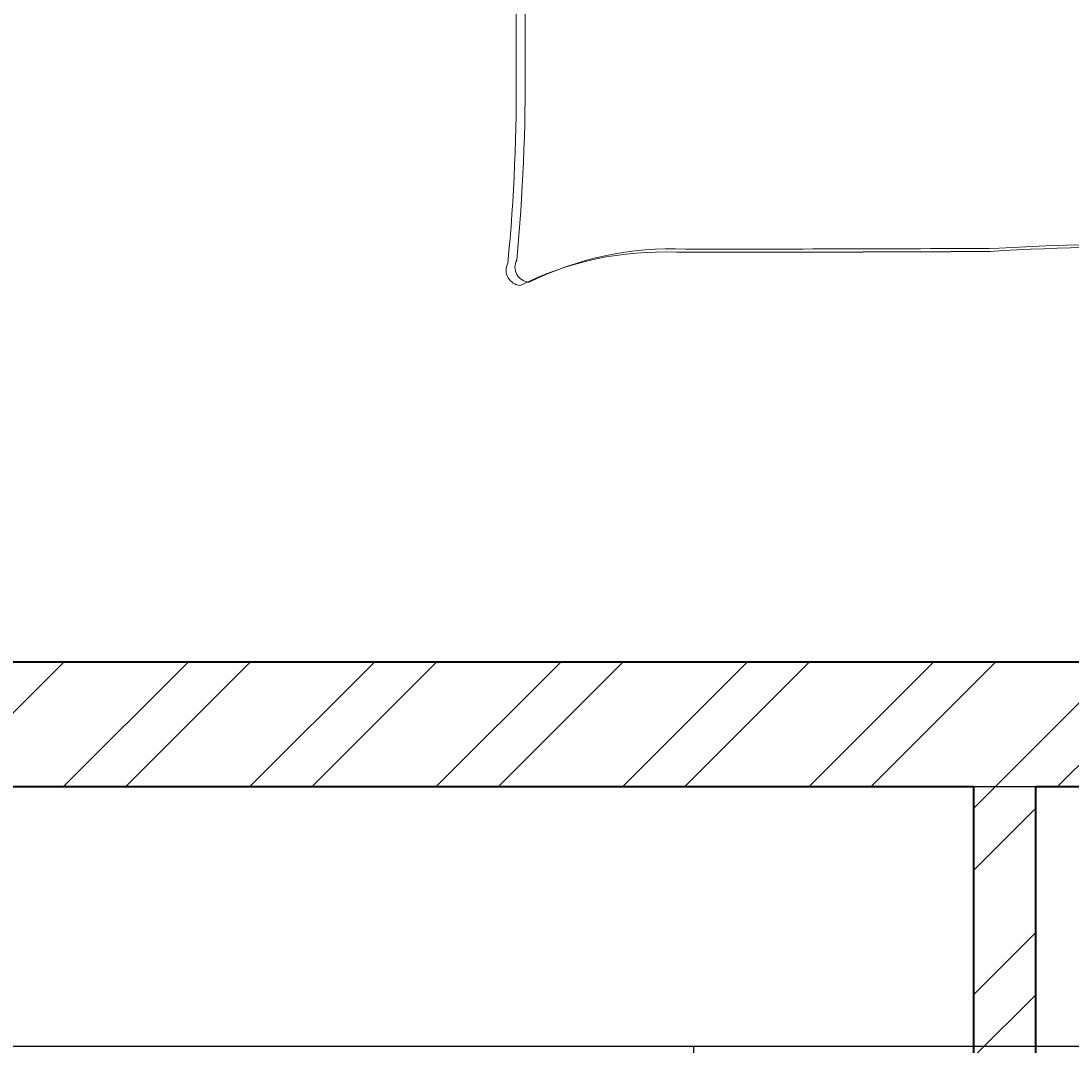
# Model space of a CAD drawing. Units: inches. Extents: x 1601 to 2297, y 1496 to 2631.
# Tile 29 of 57: x 2109 to 2185, y 2067 to 2141. Entities that reach past the tile are written whole.
import ezdxf

# ---------------------------------------------------------------- set-up
doc = ezdxf.new("R2010")
doc.units = ezdxf.units.IN
for name, color, linetype, lineweight in [('A-ANNO-DIMS', 2, 'Continuous', 18), ('A-FURN', 8, 'Continuous', 18), ('A-WALL', 7, 'Continuous', 40), ('A-WALL-PATT', 215, 'Continuous', 13)]:
    doc.layers.add(name, color=color, linetype=linetype, lineweight=lineweight)
doc.styles.get("Standard").update_dxf_attribs({"font": 'arial.ttf'})
doc.dimstyles.get("Standard").update_dxf_attribs({"dimtxt": 0.18, "dimasz": 0.18, "dimexe": 0.18, "dimexo": 0.0625, "dimgap": 0.09, "dimtad": 0, "dimtih": 1, "dimtoh": 1, "dimdec": 4, "dimzin": 0, "dimdsep": 46, "dimtxsty": 'Standard', "dimcen": 0.09, "dimadec": 0, "dimazin": 0, "dimtfac": 1, "dimtdec": 4, "dimtofl": 0, "dimtmove": 0, "dimatfit": 3, "dimfxl": 1, "dimtolj": 1, "dimtzin": 0, "dimarcsym": 0})

# ---------------------------------------------------------------- blocks, each defined once
blk = doc.blocks.new('BED-DOUBLE')
for p, q in [((30.13, 53.175), (28.385, 53.096, 3.871)), ((30.13, 53.175), (28.385, 53.096, 3.871)), ((30.13, 53.175), (28.385, 53.096, 3.871)), ((30.13, 53.175), (28.385, 53.096, 3.871)), ((27.746, 52.867), (24.495, 49.162)), ((27.746, 52.867), (24.495, 49.162)), ((27.746, 52.867), (24.495, 49.162)), ((27.746, 52.867), (24.495, 49.162)), ((28.385, 53.096), (25.135, 49.39)), ((28.385, 53.096), (25.135, 49.39)), ((28.385, 53.096), (25.135, 49.39)), ((28.385, 53.096), (25.135, 49.39)), ((29.49, 52.947), (27.746, 52.867, 3.871)), ((29.49, 52.947), (27.746, 52.867, 3.871)), ((29.49, 52.947), (27.746, 52.867, 3.871)), ((29.49, 52.947), (27.746, 52.867, 3.871)), ((28.365, 51.33), (27.746, 52.867)), ((28.365, 51.33), (27.746, 52.867)), ((28.365, 51.33), (27.746, 52.867)), ((28.365, 51.33), (27.746, 52.867)), ((29.004, 51.559), (28.385, 53.096)), ((29.004, 51.558), (28.385, 53.096)), ((29.004, 51.559), (28.385, 53.096)), ((29.004, 51.558), (28.385, 53.096)), ((0, 51.494), (0.639, 51.493)), ((0, 3.475), (0, 51.494)), ((0, 51.494), (0.639, 51.493)), ((0, 3.475), (0, 51.494)), ((0, 51.265), (26.61, 51.265)), ((0, 51.265), (26.61, 51.265)), ((0, 51.265), (26.61, 51.265)), ((0, 51.265), (26.61, 51.265)), ((0.639, 51.494), (27.249, 51.494)), ((0.639, 51.494), (27.249, 51.494)), ((0.639, 51.493), (27.249, 51.493)), ((0.639, 51.493), (27.249, 51.493)), ((1.533, 3.475), (1.533, 51.265)), ((1.533, 3.475), (1.533, 51.265)), ((1.533, 3.475), (1.533, 51.265)), ((1.533, 3.475), (1.533, 51.265)), ((2.173, 3.703), (2.173, 51.494)), ((2.173, 3.703), (2.173, 51.494)), ((2.173, 3.703), (2.173, 51.493)), ((2.173, 3.703), (2.173, 51.493)), ((17.212, 50.926), (14.073, 50.151)), ((17.212, 50.926), (14.073, 50.151)), ((17.212, 50.926), (14.073, 50.151)), ((17.212, 50.926), (14.073, 50.151)), ((16.808, 45.795), (17.212, 50.926)), ((16.808, 45.794), (17.212, 50.926)), ((16.808, 45.795), (17.212, 50.926)), ((16.808, 45.794), (17.212, 50.926)), ((28.055, 48.233), (28.365, 51.33)), ((28.055, 48.233), (28.365, 51.33)), ((28.055, 48.233), (28.365, 51.33)), ((28.055, 48.233), (28.365, 51.33)), ((28.695, 48.461), (29.004, 51.559)), ((28.695, 48.461), (29.004, 51.559)), ((28.695, 48.461), (29.004, 51.558)), ((28.695, 48.461), (29.004, 51.558)), ((2.557, 50.112), (2.46, 44.709)), ((2.557, 50.112), (2.46, 44.709)), ((2.557, 50.111), (2.46, 44.709)), ((2.557, 50.111), (2.46, 44.709)), ((2.557, 50.112), (5.768, 49.733)), ((2.557, 50.112), (5.768, 49.733)), ((2.557, 50.111), (5.768, 49.733)), ((2.557, 50.111), (5.768, 49.733)), ((3.196, 50.34), (3.099, 44.938)), ((3.196, 50.34), (3.099, 44.938)), ((3.196, 50.34), (3.099, 44.938)), ((3.196, 50.34), (3.099, 44.938)), ((3.196, 50.34), (6.407, 49.961)), ((3.196, 50.34), (6.407, 49.961)), ((3.196, 50.34), (6.407, 49.961)), ((3.196, 50.34), (6.407, 49.961)), ((5.768, 49.733), (8.338, 50.328)), ((5.768, 49.733), (8.338, 50.328)), ((5.768, 49.733), (8.338, 50.328)), ((5.768, 49.733), (8.338, 50.328)), ((6.407, 49.961), (8.977, 50.557)), ((6.407, 49.961), (8.977, 50.557)), ((6.407, 49.961), (8.977, 50.556)), ((6.407, 49.961), (8.977, 50.556)), ((11.829, 50.112), (8.257, 49.309)), ((11.829, 50.112), (8.257, 49.309)), ((11.829, 50.112), (8.257, 49.309)), ((11.829, 50.112), (8.257, 49.309)), ((8.338, 50.328), (9.384, 49.814)), ((8.338, 50.328), (9.384, 49.814)), ((8.338, 50.328), (9.384, 49.814)), ((8.338, 50.328), (9.384, 49.814)), ((12.468, 50.34), (8.896, 49.538)), ((12.468, 50.34), (8.896, 49.537)), ((12.468, 50.34), (8.896, 49.538)), ((12.468, 50.34), (8.896, 49.537)), ((8.977, 50.557), (10.024, 50.043)), ((8.977, 50.557), (10.024, 50.043)), ((8.977, 50.556), (10.024, 50.042)), ((8.977, 50.556), (10.024, 50.042)), ((13.434, 49.923), (11.829, 50.112)), ((13.434, 49.922), (11.829, 50.112)), ((13.434, 49.923), (11.829, 50.112)), ((13.434, 49.922), (11.829, 50.112)), ((14.073, 50.151), (12.468, 50.34)), ((14.073, 50.151), (12.468, 50.34)), ((14.073, 50.151), (12.468, 50.34)), ((14.073, 50.151), (12.468, 50.34)), ((16.573, 50.698), (13.434, 49.923)), ((16.573, 50.698), (13.434, 49.922)), ((16.573, 50.698), (13.434, 49.923)), ((16.573, 50.698), (13.434, 49.922)), ((16.169, 45.566), (16.573, 50.698)), ((16.169, 45.566), (16.573, 50.698)), ((16.169, 45.566), (16.573, 50.698)), ((16.169, 45.566), (16.573, 50.698)), ((8.896, 49.538), (6.218, 48.356)), ((8.896, 49.538), (6.218, 48.356)), ((8.896, 49.537), (6.218, 48.356)), ((8.896, 49.537), (6.218, 48.356)), ((25.135, 49.39), (22.968, 46.448)), ((25.135, 49.39), (22.968, 46.448)), ((25.135, 49.39), (22.968, 46.448)), ((25.135, 49.39), (22.968, 46.448)), ((8.257, 49.309), (5.578, 48.128)), ((8.257, 49.309), (5.578, 48.128)), ((8.257, 49.309), (5.578, 48.128)), ((8.257, 49.309), (5.578, 48.128)), ((24.495, 49.162), (22.329, 46.219)), ((24.495, 49.162), (22.329, 46.219)), ((24.495, 49.162), (22.329, 46.219)), ((24.495, 49.162), (22.329, 46.219)), ((28.365, 44.361), (28.055, 48.233)), ((28.365, 44.361), (28.055, 48.233)), ((28.365, 44.361), (28.055, 48.233)), ((28.365, 44.361), (28.055, 48.233)), ((29.004, 44.589), (28.695, 48.461)), ((29.004, 44.589), (28.695, 48.461)), ((29.004, 44.589), (28.695, 48.461)), ((29.004, 44.589), (28.695, 48.461)), ((22.968, 46.448), (20.956, 40.872)), ((22.968, 46.448), (20.956, 40.872)), ((22.968, 46.448), (20.956, 40.872)), ((22.968, 46.448), (20.956, 40.872)), ((2.46, 44.709), (2.542, 45.712)), ((2.46, 44.709), (2.542, 45.712)), ((2.46, 44.709), (2.542, 45.712)), ((2.46, 44.709), (2.542, 45.712)), ((2.542, 45.712), (3.069, 41.914)), ((2.542, 45.712), (3.069, 41.914)), ((2.542, 45.712), (3.069, 41.914)), ((2.542, 45.712), (3.069, 41.914)), ((3.099, 44.938), (3.181, 45.941)), ((3.099, 44.938), (3.181, 45.941)), ((3.099, 44.938), (3.181, 45.94)), ((3.099, 44.938), (3.181, 45.94)), ((3.181, 45.941), (3.709, 42.143)), ((3.181, 45.941), (3.709, 42.143)), ((3.181, 45.94), (3.709, 42.142)), ((3.181, 45.94), (3.709, 42.142)), ((16.726, 43.606), (16.169, 45.566)), ((16.726, 43.606), (16.169, 45.566)), ((16.726, 43.606), (16.169, 45.566)), ((16.726, 43.606), (16.169, 45.566)), ((17.365, 43.834), (16.808, 45.795)), ((17.365, 43.834), (16.808, 45.795)), ((17.365, 43.834), (16.808, 45.794)), ((17.365, 43.834), (16.808, 45.794)), ((22.329, 46.219), (20.316, 40.644)), ((22.329, 46.219), (20.316, 40.644)), ((22.329, 46.219), (20.317, 40.644)), ((22.329, 46.219), (20.317, 40.644)), ((28.829, 40.954), (28.365, 44.361)), ((28.829, 40.953), (28.365, 44.361)), ((28.829, 40.954), (28.365, 44.361)), ((28.829, 40.953), (28.365, 44.361)), ((29.468, 41.182), (29.004, 44.589)), ((29.469, 41.182), (29.004, 44.589)), ((29.468, 41.182), (29.004, 44.589)), ((29.469, 41.182), (29.004, 44.589)), ((16.295, 36.596), (16.726, 43.606)), ((16.295, 36.596), (16.726, 43.606)), ((16.295, 36.596), (16.726, 43.606)), ((16.295, 36.596), (16.726, 43.606)), ((16.934, 36.824), (17.365, 43.834)), ((16.934, 36.824), (17.365, 43.834)), ((16.934, 36.824), (17.365, 43.834)), ((16.934, 36.824), (17.365, 43.834)), ((3.069, 41.914), (4.422, 36.495)), ((3.069, 41.914), (4.422, 36.495)), ((3.069, 41.914), (4.422, 36.495)), ((3.069, 41.914), (4.422, 36.495)), ((3.709, 42.143), (5.061, 36.723)), ((3.709, 42.143), (5.061, 36.723)), ((3.709, 42.142), (5.061, 36.723)), ((3.709, 42.142), (5.061, 36.723)), ((30.397, 39.169), (29.468, 41.182)), ((30.397, 39.169), (29.468, 41.182)), ((30.397, 39.168), (29.469, 41.182)), ((30.397, 39.168), (29.469, 41.182)), ((20.316, 40.644), (17.383, 32.306)), ((20.317, 40.644), (17.383, 32.306)), ((20.316, 40.644), (17.383, 32.306)), ((20.317, 40.644), (17.383, 32.306)), ((20.956, 40.872), (18.022, 32.534)), ((20.956, 40.872), (18.022, 32.534)), ((20.956, 40.872), (18.022, 32.534)), ((20.956, 40.872), (18.022, 32.534)), ((29.758, 38.94), (28.829, 40.954)), ((29.758, 38.94), (28.829, 40.954)), ((29.758, 38.94), (28.829, 40.953)), ((29.758, 38.94), (28.829, 40.953)), ((79.245, 15.063), (79.245, 39.677)), ((79.245, 15.063), (79.245, 39.677)), ((79.245, 15.063), (79.245, 39.677)), ((79.245, 15.063), (79.245, 39.677)), ((79.884, 15.292), (79.884, 39.905)), ((79.884, 15.291), (79.884, 39.905)), ((79.884, 15.292), (79.884, 39.905)), ((79.884, 15.291), (79.884, 39.905)), ((3.673, 39.2), (3.078, 37.135)), ((3.673, 39.2), (3.078, 37.135)), ((3.673, 39.2), (3.078, 37.135)), ((3.673, 39.2), (3.078, 37.135)), ((4.313, 39.428), (3.717, 37.363)), ((4.313, 39.428), (3.717, 37.363)), ((4.313, 39.428), (3.718, 37.363)), ((4.313, 39.428), (3.718, 37.363)), ((30.377, 36.462), (29.758, 38.94)), ((30.377, 36.462), (29.758, 38.94)), ((30.377, 36.462), (29.758, 38.94)), ((30.377, 36.462), (29.758, 38.94)), ((31.016, 36.691), (30.397, 39.169)), ((31.016, 36.691), (30.397, 39.169)), ((31.016, 36.691), (30.397, 39.168)), ((31.016, 36.691), (30.397, 39.168)), ((3.717, 37.363), (3.176, 34.433)), ((3.718, 37.363), (3.176, 34.433)), ((3.717, 37.363), (3.176, 34.433)), ((3.718, 37.363), (3.176, 34.433)), ((3.078, 37.135), (2.537, 34.204)), ((3.078, 37.135), (2.537, 34.204)), ((3.078, 37.135), (2.537, 34.204)), ((3.078, 37.135), (2.537, 34.204)), ((15.628, 32.564), (16.295, 36.596)), ((15.628, 32.564), (16.295, 36.596)), ((15.628, 32.564), (16.295, 36.596)), ((15.628, 32.564), (16.295, 36.596)), ((16.268, 32.792), (16.934, 36.824)), ((16.268, 32.792), (16.934, 36.824)), ((16.268, 32.792), (16.934, 36.824)), ((16.268, 32.792), (16.934, 36.824)), ((28.365, 36.153), (30.377, 36.462)), ((28.365, 36.152), (30.377, 36.462)), ((28.365, 36.153), (30.377, 36.462)), ((28.365, 36.152), (30.377, 36.462)), ((29.004, 36.381), (31.016, 36.691)), ((29.004, 36.381), (31.016, 36.691)), ((29.004, 36.381), (31.016, 36.691)), ((29.004, 36.381), (31.016, 36.691)), ((23.876, 34.449), (28.365, 36.153)), ((23.876, 34.449), (28.365, 36.153)), ((23.876, 34.449), (28.365, 36.152)), ((23.876, 34.449), (28.365, 36.152)), ((24.516, 34.677), (29.004, 36.381)), ((24.516, 34.677), (29.004, 36.381)), ((24.516, 34.677), (29.004, 36.381)), ((24.516, 34.677), (29.004, 36.381)), ((2.537, 34.204), (2.557, 33.883)), ((2.537, 34.204), (2.557, 33.883)), ((2.537, 34.204), (2.557, 33.883)), ((2.537, 34.204), (2.557, 33.883)), ((3.176, 34.433), (3.196, 34.112)), ((3.176, 34.433), (3.196, 34.112)), ((3.176, 34.433), (3.196, 34.112)), ((3.176, 34.433), (3.196, 34.112)), ((17.383, 30.259), (23.876, 34.449)), ((17.383, 30.259), (23.876, 34.449)), ((17.383, 30.259), (23.876, 34.449)), ((17.383, 30.259), (23.876, 34.449)), ((18.022, 30.487), (24.516, 34.677)), ((18.022, 30.487), (24.516, 34.677)), ((18.022, 30.487), (24.516, 34.677)), ((18.022, 30.487), (24.516, 34.677)), ((2.557, 33.883), (2.979, 29.456)), ((2.557, 33.883), (2.979, 29.455)), ((2.557, 33.883), (2.979, 29.456)), ((2.557, 33.883), (2.979, 29.455)), ((3.196, 34.112), (3.618, 29.684)), ((3.196, 34.112), (3.618, 29.684)), ((3.196, 34.112), (3.618, 29.684)), ((3.196, 34.112), (3.618, 29.684)), ((16.739, 30.75), (15.454, 33.821)), ((16.739, 30.75), (15.454, 33.821)), ((16.739, 30.75), (15.454, 33.82)), ((16.739, 30.75), (15.454, 33.82)), ((17.379, 30.978), (16.094, 34.049)), ((17.379, 30.978), (16.094, 34.049)), ((17.379, 30.978), (16.094, 34.049)), ((17.379, 30.978), (16.094, 34.049)), ((16.893, 28.297), (16.739, 30.75)), ((16.893, 28.297), (16.739, 30.75)), ((16.893, 28.297), (16.739, 30.75)), ((16.893, 28.297), (16.739, 30.75)), ((17.532, 28.526), (17.379, 30.978)), ((17.532, 28.525), (17.379, 30.978)), ((17.532, 28.526), (17.379, 30.978)), ((17.532, 28.525), (17.379, 30.978)), ((3.618, 29.684), (3.131, 28.205)), ((3.618, 29.684), (3.131, 28.205)), ((3.618, 29.684), (3.131, 28.205)), ((3.618, 29.684), (3.131, 28.205)), ((2.979, 29.456), (2.492, 27.977)), ((2.979, 29.456), (2.492, 27.977)), ((2.979, 29.455), (2.492, 27.976)), ((2.979, 29.455), (2.492, 27.976)), ((3.131, 28.205), (8.506, 27.962)), ((3.131, 28.205), (8.506, 27.961)), ((3.131, 28.205), (8.506, 27.962)), ((3.131, 28.205), (8.506, 27.961)), ((12.377, 27.436), (14.216, 28.13)), ((12.377, 27.436), (14.217, 28.13)), ((12.377, 27.436), (14.216, 28.13)), ((12.377, 27.436), (14.217, 28.13)), ((13.016, 27.664), (14.856, 28.359)), ((13.016, 27.664), (14.856, 28.359)), ((13.016, 27.664), (14.856, 28.358)), ((13.016, 27.664), (14.856, 28.358)), ((14.216, 28.13), (16.893, 28.297)), ((14.216, 28.13), (16.893, 28.297)), ((14.217, 28.13), (16.893, 28.297)), ((14.217, 28.13), (16.893, 28.297)), ((14.856, 28.359), (17.532, 28.526)), ((14.856, 28.359), (17.532, 28.526)), ((14.856, 28.358), (17.532, 28.525)), ((14.856, 28.358), (17.532, 28.525)), ((2.492, 27.977), (7.867, 27.733)), ((2.492, 27.977), (7.867, 27.733)), ((2.492, 27.976), (7.867, 27.733)), ((2.492, 27.976), (7.867, 27.733)), ((7.859, 26.789), (11.04, 27.367)), ((7.859, 26.789), (11.04, 27.367)), ((7.859, 26.789), (11.04, 27.367)), ((7.859, 26.789), (11.04, 27.367)), ((7.867, 27.733), (11.078, 27.355)), ((7.867, 27.733), (11.078, 27.354)), ((7.867, 27.733), (11.078, 27.355)), ((7.867, 27.733), (11.078, 27.354)), ((8.506, 27.962), (11.717, 27.583)), ((8.506, 27.962), (11.717, 27.583)), ((8.506, 27.961), (11.717, 27.583)), ((8.506, 27.961), (11.717, 27.583)), ((11.04, 27.367), (12.341, 27.367)), ((11.04, 27.367), (12.341, 27.367)), ((11.04, 27.367), (12.341, 27.367)), ((11.04, 27.367), (12.341, 27.367)), ((11.078, 27.355), (12.377, 27.436)), ((11.078, 27.354), (12.377, 27.436)), ((11.078, 27.355), (12.377, 27.436)), ((11.078, 27.354), (12.377, 27.436)), ((11.717, 27.583), (13.016, 27.664)), ((11.717, 27.583), (13.016, 27.664)), ((11.717, 27.583), (13.016, 27.664)), ((11.717, 27.583), (13.016, 27.664)), ((12.341, 27.367), (14.221, 26.789)), ((12.341, 27.367), (14.221, 26.789)), ((12.341, 27.367), (14.221, 26.789)), ((12.341, 27.367), (14.221, 26.789)), ((2.509, 26.211), (7.859, 26.789)), ((2.509, 26.21), (7.859, 26.789)), ((2.509, 26.211), (7.859, 26.789)), ((2.509, 26.21), (7.859, 26.789)), ((7.22, 26.561), (10.401, 27.139)), ((7.22, 26.56), (10.401, 27.139)), ((7.22, 26.561), (10.401, 27.139)), ((7.22, 26.56), (10.401, 27.139)), ((10.401, 27.139), (11.702, 27.139)), ((10.401, 27.139), (11.702, 27.139)), ((10.401, 27.139), (11.702, 27.139)), ((10.401, 27.139), (11.702, 27.139)), ((11.702, 27.139), (13.582, 26.561)), ((11.702, 27.139), (13.582, 26.56)), ((11.702, 27.139), (13.582, 26.561)), ((11.702, 27.139), (13.582, 26.56)), ((14.221, 26.789), (16.902, 26.789)), ((14.221, 26.789), (16.902, 26.789)), ((14.221, 26.789), (16.902, 26.789)), ((14.221, 26.789), (16.902, 26.789)), ((16.902, 26.789), (16.902, 24.332)), ((16.902, 26.789), (16.902, 24.331)), ((16.902, 26.789), (16.902, 24.332)), ((16.902, 26.789), (16.902, 24.331)), ((1.87, 25.982), (7.22, 26.561)), ((1.87, 25.982), (7.22, 26.561)), ((1.87, 25.982), (7.22, 26.56)), ((1.87, 25.982), (7.22, 26.56)), ((2.448, 24.537), (1.87, 25.982)), ((2.448, 24.537), (1.87, 25.982)), ((2.448, 24.537), (1.87, 25.982)), ((2.448, 24.537), (1.87, 25.982)), ((3.088, 24.765), (2.509, 26.211)), ((3.088, 24.765), (2.509, 26.211)), ((3.088, 24.765), (2.509, 26.21)), ((3.088, 24.765), (2.509, 26.21)), ((13.582, 26.561), (16.263, 26.561)), ((13.582, 26.561), (16.263, 26.561)), ((13.582, 26.56), (16.263, 26.56)), ((13.582, 26.56), (16.263, 26.56)), ((16.263, 26.561), (16.263, 24.103)), ((16.263, 26.561), (16.263, 24.103)), ((16.263, 26.56), (16.263, 24.103)), ((16.263, 26.56), (16.263, 24.103)), ((2.304, 20.091), (2.448, 24.537)), ((2.304, 20.091), (2.448, 24.537)), ((2.304, 20.091), (2.448, 24.537)), ((2.304, 20.091), (2.448, 24.537)), ((2.943, 20.32), (3.088, 24.765)), ((2.943, 20.319), (3.088, 24.765)), ((2.943, 20.32), (3.088, 24.765)), ((2.943, 20.319), (3.088, 24.765)), ((16.902, 24.332), (15.811, 21.187)), ((16.902, 24.332), (15.811, 21.187)), ((16.902, 24.331), (15.811, 21.187)), ((16.902, 24.331), (15.811, 21.187)), ((16.169, 19.384), (16.573, 24.516)), ((16.169, 19.384), (16.573, 24.516)), ((16.169, 19.383), (16.573, 24.515)), ((16.169, 19.383), (16.573, 24.515)), ((16.808, 19.612), (17.212, 24.744)), ((16.808, 19.612), (17.212, 24.744)), ((16.808, 19.612), (17.212, 24.744)), ((16.808, 19.612), (17.212, 24.744)), ((16.263, 24.103), (15.172, 20.959)), ((16.263, 24.103), (15.172, 20.958)), ((16.263, 24.103), (15.172, 20.959)), ((16.263, 24.103), (15.172, 20.958)), ((2.304, 19.77), (2.304, 20.091)), ((2.304, 19.769), (2.304, 20.091)), ((2.304, 19.77), (2.304, 20.091)), ((2.304, 19.769), (2.304, 20.091)), ((3.027, 16.878), (2.304, 19.77)), ((3.027, 16.878), (2.304, 19.77)), ((3.027, 16.878), (2.304, 19.769)), ((3.027, 16.878), (2.304, 19.769)), ((2.943, 19.998), (2.943, 20.32)), ((2.943, 19.998), (2.943, 20.32)), ((2.943, 19.998), (2.943, 20.319)), ((2.943, 19.998), (2.943, 20.319)), ((3.666, 17.107), (2.943, 19.998)), ((3.666, 17.107), (2.943, 19.998)), ((3.666, 17.107), (2.943, 19.998)), ((3.666, 17.107), (2.943, 19.998)), ((16.726, 17.423), (16.169, 19.384)), ((16.726, 17.423), (16.169, 19.384)), ((16.726, 17.423), (16.169, 19.383)), ((16.726, 17.423), (16.169, 19.383)), ((17.365, 17.652), (16.808, 19.612)), ((17.365, 17.651), (16.808, 19.612)), ((17.365, 17.652), (16.808, 19.612)), ((17.365, 17.651), (16.808, 19.612)), ((3.316, 12.108), (4.328, 17.601)), ((3.316, 12.108), (4.328, 17.601)), ((3.316, 12.108), (4.328, 17.601)), ((3.316, 12.108), (4.328, 17.601)), ((3.955, 12.336), (4.967, 17.83)), ((3.955, 12.336), (4.967, 17.83)), ((3.955, 12.336), (4.967, 17.829)), ((3.955, 12.336), (4.967, 17.829)), ((16.934, 10.642), (17.365, 17.652)), ((16.934, 10.642), (17.365, 17.652)), ((16.934, 10.642), (17.365, 17.651)), ((16.934, 10.642), (17.365, 17.651)), ((3.75, 14.855), (3.027, 16.878)), ((3.75, 14.854), (3.027, 16.878)), ((3.75, 14.855), (3.027, 16.878)), ((3.75, 14.854), (3.027, 16.878)), ((4.389, 15.083), (3.666, 17.107)), ((4.389, 15.083), (3.666, 17.107)), ((4.389, 15.083), (3.666, 17.107)), ((4.389, 15.083), (3.666, 17.107)), ((16.295, 10.413), (16.726, 17.423)), ((16.295, 10.413), (16.726, 17.423)), ((16.295, 10.413), (16.726, 17.423)), ((16.295, 10.413), (16.726, 17.423)), ((3.666, 8.513), (3.955, 12.336)), ((3.666, 8.513), (3.955, 12.336)), ((3.666, 8.513), (3.955, 12.336)), ((3.666, 8.513), (3.955, 12.336)), ((3.027, 8.285), (3.316, 12.108)), ((3.027, 8.284), (3.316, 12.108)), ((3.027, 8.285), (3.316, 12.108)), ((3.027, 8.284), (3.316, 12.108)), ((16.268, 6.61), (16.934, 10.642)), ((16.268, 6.61), (16.934, 10.642)), ((16.268, 6.61), (16.934, 10.642)), ((16.268, 6.61), (16.934, 10.642)), ((16.934, 10.642), (17.257, 9.509)), ((16.934, 10.642), (17.257, 9.508)), ((16.934, 10.642), (17.257, 9.509)), ((16.934, 10.642), (17.257, 9.508)), ((15.628, 6.382), (16.295, 10.413)), ((15.628, 6.381), (16.295, 10.413)), ((15.628, 6.382), (16.295, 10.413)), ((15.628, 6.381), (16.295, 10.413)), ((16.295, 10.413), (16.618, 9.28)), ((16.295, 10.413), (16.618, 9.28)), ((16.295, 10.413), (16.618, 9.28)), ((16.295, 10.413), (16.618, 9.28)), ((16.618, 9.28), (17.341, 4.184)), ((16.618, 9.28), (17.341, 4.183)), ((16.618, 9.28), (17.341, 4.184)), ((16.618, 9.28), (17.341, 4.183)), ((17.257, 9.509), (17.98, 4.412)), ((17.257, 9.509), (17.98, 4.412)), ((17.257, 9.508), (17.98, 4.412)), ((17.257, 9.508), (17.98, 4.412)), ((3.648, 8.408), (3.666, 8.513)), ((3.648, 8.407), (3.666, 8.513)), ((3.648, 8.408), (3.666, 8.513)), ((3.648, 8.407), (3.666, 8.513)), ((3.977, 4.127), (3.648, 8.408)), ((3.977, 4.127), (3.648, 8.408)), ((3.977, 4.127), (3.648, 8.407)), ((3.977, 4.127), (3.648, 8.407)), ((3.009, 8.179), (3.027, 8.285)), ((3.009, 8.179), (3.027, 8.285)), ((3.009, 8.179), (3.027, 8.284)), ((3.009, 8.179), (3.027, 8.284)), ((3.338, 3.898), (3.009, 8.179)), ((3.338, 3.898), (3.009, 8.179)), ((3.338, 3.898), (3.009, 8.179)), ((3.338, 3.898), (3.009, 8.179)), ((9.594, 5.279), (6.847, 6.291)), ((9.594, 5.279), (6.847, 6.291)), ((9.594, 5.279), (6.847, 6.291)), ((9.594, 5.279), (6.847, 6.291)), ((8.955, 5.051), (6.208, 6.063)), ((8.955, 5.051), (6.208, 6.063)), ((8.955, 5.051), (6.208, 6.063)), ((8.955, 5.051), (6.208, 6.063)), ((3.955, 4.123), (7.136, 4.701)), ((3.955, 4.123), (7.136, 4.701)), ((3.955, 4.123), (7.136, 4.701)), ((3.955, 4.123), (7.136, 4.701)), ((7.136, 4.701), (9.739, 4.267)), ((7.136, 4.701), (9.739, 4.267)), ((7.136, 4.701), (9.739, 4.267)), ((7.136, 4.701), (9.739, 4.267)), ((12.57, 4.473), (8.955, 5.051)), ((12.57, 4.472), (8.955, 5.051)), ((12.57, 4.473), (8.955, 5.051)), ((12.57, 4.472), (8.955, 5.051)), ((9.099, 4.039), (10.112, 4.617)), ((9.099, 4.039), (10.112, 4.617)), ((9.099, 4.039), (10.112, 4.617)), ((9.099, 4.039), (10.112, 4.617)), ((13.209, 4.701), (9.594, 5.279)), ((13.209, 4.701), (9.594, 5.279)), ((13.209, 4.701), (9.594, 5.279)), ((13.209, 4.701), (9.594, 5.279)), ((9.739, 4.267), (10.751, 4.846)), ((9.739, 4.267), (10.751, 4.846)), ((9.739, 4.267), (10.751, 4.845)), ((9.739, 4.267), (10.751, 4.845)), ((14.16, 4.762), (12.57, 4.473)), ((14.16, 4.762), (12.57, 4.472)), ((14.16, 4.762), (12.57, 4.473)), ((14.16, 4.762), (12.57, 4.472)), ((14.799, 4.99), (13.209, 4.701)), ((14.799, 4.99), (13.209, 4.701)), ((14.799, 4.99), (13.209, 4.701)), ((14.799, 4.99), (13.209, 4.701)), ((17.341, 4.184), (14.16, 4.762)), ((17.341, 4.183), (14.16, 4.762)), ((17.341, 4.184), (14.16, 4.762)), ((17.341, 4.183), (14.16, 4.762)), ((17.98, 4.412), (14.799, 4.99)), ((17.98, 4.412), (14.799, 4.99)), ((17.98, 4.412), (14.799, 4.99)), ((17.98, 4.412), (14.799, 4.99)), ((3.316, 3.894), (6.497, 4.473)), ((3.316, 3.894), (6.497, 4.473)), ((3.316, 3.894), (6.497, 4.472)), ((3.316, 3.894), (6.497, 4.472)), ((6.497, 4.473), (9.099, 4.039)), ((6.497, 4.473), (9.099, 4.039)), ((6.497, 4.472), (9.099, 4.039)), ((6.497, 4.472), (9.099, 4.039)), ((18.11, 3.475), (0, 3.475)), ((18.11, 3.475), (0, 3.475)), ((18.11, 3.475), (0, 3.475)), ((18.11, 3.475), (0, 3.475)), ((18.75, 3.703), (0.639, 3.703)), ((18.75, 3.703), (0.639, 3.703)), ((18.75, 3.703), (0.639, 3.703)), ((18.75, 3.703), (0.639, 3.703))]:
    blk.add_line(p, q)
for centre, radius, start, end in [((68.666, 76.157), 23.065, 267.47136, 296.46809), ((68.666, 76.157), 23.065, 267.47136, 296.46809), ((68.666, 76.157), 23.065, 267.47136, 296.46809), ((68.666, 76.157), 23.065, 267.47136, 296.46809), ((69.306, 76.385), 23.065, 267.47136, 296.46809), ((69.306, 76.385), 23.065, 267.47136, 296.46809), ((69.306, 76.385), 23.065, 267.47136, 296.46809), ((69.306, 76.385), 23.065, 267.47136, 296.46809), ((78.87, 54.41), 1.102, 332.65876, 86.02002), ((78.87, 54.409), 1.102, 332.65876, 86.02002), ((78.87, 54.41), 1.102, 332.65876, 86.02002), ((78.87, 54.409), 1.102, 332.65876, 86.02002), ((79.509, 54.638), 1.102, 332.65876, 86.02002), ((79.509, 54.638), 1.102, 332.65876, 86.02002), ((79.509, 54.638), 1.102, 332.65876, 86.02002), ((79.509, 54.638), 1.102, 332.65876, 86.02002), ((212.276, 41.152), 133.04, 174.4998, 180.63509), ((212.277, 41.151), 133.04, 174.4998, 180.63509), ((212.276, 41.152), 133.04, 174.4998, 180.63509), ((212.277, 41.151), 133.04, 174.4998, 180.63509), ((212.916, 41.38), 133.04, 174.4998, 180.63509), ((212.916, 41.38), 133.04, 174.4998, 180.63509), ((212.916, 41.38), 133.04, 174.4998, 180.63509), ((212.916, 41.38), 133.04, 174.4998, 180.63509), ((-6.017, 51.555), 36.183, 349.87628, 2.56571), ((-6.017, 51.555), 36.183, 349.87628, 2.56571), ((-6.017, 51.555), 36.183, 349.87628, 2.56571), ((-6.017, 51.555), 36.183, 349.87628, 2.56571), ((36.954, 182.494), 129.499, 266.97912, 273.83645), ((36.954, 182.494), 129.499, 266.97912, 273.83645), ((36.954, 182.494), 129.499, 266.97912, 273.83645), ((36.954, 182.494), 129.499, 266.97912, 273.83645), ((68.461, -4508.515), 4561.858, 90.002168, 90.286887), ((68.461, -4508.515), 4561.858, 90.002168, 90.286887), ((68.461, -4508.516), 4561.858, 90.002168, 90.286887), ((68.461, -4508.516), 4561.858, 90.002168, 90.286887), ((-6.656, 51.327), 36.183, 349.87628, 2.56571), ((-6.656, 51.327), 36.183, 349.87628, 2.56571), ((-6.656, 51.327), 36.183, 349.87628, 2.56571), ((-6.656, 51.327), 36.183, 349.87628, 2.56571), ((36.315, 182.266), 129.499, 266.97912, 273.83645), ((36.315, 182.265), 129.499, 266.97912, 273.83645), ((36.315, 182.266), 129.499, 266.97912, 273.83645), ((36.315, 182.265), 129.499, 266.97912, 273.83645), ((67.821, -4508.744), 4561.858, 90.002168, 90.286887), ((67.821, -4508.744), 4561.858, 90.002168, 90.286887), ((67.821, -4508.744), 4561.858, 90.002168, 90.286887), ((67.821, -4508.744), 4561.858, 90.002168, 90.286887), ((35.066, 43.743), 6.224, 168.6608, 203.73842), ((35.066, 43.743), 6.224, 168.6608, 203.73842), ((35.066, 43.743), 6.224, 168.6608, 203.73842), ((35.066, 43.743), 6.224, 168.6608, 203.73842), ((35.705, 43.972), 6.224, 168.6608, 203.73842), ((35.705, 43.971), 6.224, 168.6608, 203.73842), ((35.705, 43.972), 6.224, 168.6608, 203.73842), ((35.705, 43.971), 6.224, 168.6608, 203.73842), ((1.482, 31.154), 29.654, 10.66171, 19.88058), ((1.482, 31.154), 29.654, 10.66171, 19.88058), ((1.482, 31.153), 29.654, 10.66171, 19.88058), ((1.482, 31.153), 29.654, 10.66171, 19.88058), ((2.121, 31.382), 29.654, 10.66171, 19.88058), ((2.121, 31.382), 29.654, 10.66171, 19.88058), ((2.121, 31.382), 29.654, 10.66171, 19.88058), ((2.121, 31.382), 29.654, 10.66171, 19.88058), ((30.439, 36.636), 0.185, 250.24637, 1.13765), ((30.439, 36.636), 0.185, 250.24637, 1.13765), ((30.439, 36.636), 0.185, 250.24637, 1.13765), ((30.439, 36.636), 0.185, 250.24637, 1.13765), ((31.079, 36.864), 0.185, 250.24637, 1.13765), ((31.079, 36.864), 0.185, 250.24637, 1.13765), ((31.079, 36.864), 0.185, 250.24637, 1.13765), ((31.079, 36.864), 0.185, 250.24637, 1.13765), ((156.316, 17.756), 129.02, 171.78449, 186.90062), ((156.316, 17.755), 129.02, 171.78449, 186.90062), ((156.316, 17.756), 129.02, 171.78449, 186.90062), ((156.316, 17.755), 129.02, 171.78449, 186.90062), ((156.955, 17.984), 129.02, 171.78449, 186.90062), ((156.955, 17.984), 129.02, 171.78449, 186.90062), ((156.955, 17.984), 129.02, 171.78449, 186.90062), ((156.955, 17.984), 129.02, 171.78449, 186.90062), ((182.692, 21.587), 164.969, 176.08655, 186.78213), ((182.692, 21.587), 164.969, 176.08655, 186.78213), ((182.692, 21.587), 164.969, 176.08655, 186.78213), ((182.692, 21.587), 164.969, 176.08655, 186.78213), ((182.052, 21.359), 164.969, 176.08655, 186.78213), ((182.052, 21.359), 164.969, 176.08655, 186.78213), ((182.052, 21.358), 164.969, 176.08655, 186.78213), ((182.052, 21.358), 164.969, 176.08655, 186.78213), ((-23.073, -16.994), 106.459, 13.38322, 17.70533), ((-23.073, -16.994), 106.459, 13.38322, 17.70533), ((-23.073, -16.994), 106.459, 13.38322, 17.70533), ((-23.073, -16.994), 106.459, 13.38322, 17.70533), ((201.476, 21.655), 121.759, 182.99578, 189.40907), ((201.476, 21.655), 121.759, 182.99578, 189.40907), ((201.476, 21.655), 121.759, 182.99578, 189.40907), ((201.476, 21.655), 121.759, 182.99578, 189.40907), ((-23.712, -17.222), 106.459, 13.38322, 17.70533), ((-23.712, -17.222), 106.459, 13.38322, 17.70533), ((-23.712, -17.222), 106.459, 13.38322, 17.70533), ((-23.712, -17.222), 106.459, 13.38322, 17.70533), ((200.837, 21.427), 121.759, 182.99578, 189.40907), ((200.837, 21.426), 121.759, 182.99578, 189.40907), ((200.837, 21.427), 121.759, 182.99578, 189.40907), ((200.837, 21.426), 121.759, 182.99578, 189.40907), ((20.735, 85.39), 83.306, 268.72178, 275.60397), ((20.735, 85.39), 83.306, 268.72178, 275.60397), ((20.736, 85.39), 83.306, 268.72178, 275.60397), ((20.736, 85.39), 83.306, 268.72178, 275.60397), ((31.174, -167.308), 170.11, 88.4762, 91.00819), ((31.174, -167.308), 170.11, 88.4762, 91.00819), ((31.174, -167.308), 170.11, 88.4762, 91.00819), ((31.174, -167.308), 170.11, 88.4762, 91.00819), ((31.813, -167.079), 170.11, 88.4762, 91.00819), ((31.813, -167.08), 170.11, 88.4762, 91.00819), ((31.813, -167.079), 170.11, 88.4762, 91.00819), ((31.813, -167.08), 170.11, 88.4762, 91.00819), ((50.614, 484.822), 482.31, 268.22771, 271.71854), ((50.614, 484.822), 482.31, 268.22771, 271.71854), ((50.614, 484.822), 482.31, 268.22771, 271.71854), ((50.614, 484.822), 482.31, 268.22771, 271.71854), ((51.253, 485.051), 482.31, 268.22771, 271.71854), ((51.253, 485.05), 482.31, 268.22771, 271.71854), ((51.253, 485.051), 482.31, 268.22771, 271.71854), ((51.253, 485.05), 482.31, 268.22771, 271.71854), ((64.515, -26.9), 29.634, 76.06484, 88.91125), ((64.515, -26.9), 29.634, 76.06484, 88.91125), ((64.515, -26.9), 29.634, 76.06484, 88.91125), ((64.515, -26.9), 29.634, 76.06484, 88.91125), ((65.154, -26.671), 29.634, 76.06484, 88.91125), ((65.154, -26.672), 29.634, 76.06484, 88.91125), ((65.154, -26.671), 29.634, 76.06484, 88.91125), ((65.154, -26.672), 29.634, 76.06484, 88.91125), ((20.096, 85.162), 83.306, 268.72178, 275.60397), ((20.096, 85.161), 83.306, 268.72178, 275.60397), ((20.096, 85.162), 83.306, 268.72178, 275.60397), ((20.096, 85.161), 83.306, 268.72178, 275.60397), ((70.276, -21.66), 23.562, 67.97508, 86.652), ((70.276, -21.66), 23.562, 67.97508, 86.652), ((70.276, -21.66), 23.562, 67.97508, 86.652), ((70.276, -21.66), 23.562, 67.97508, 86.652), ((70.915, -21.431), 23.562, 67.97508, 86.652), ((70.915, -21.432), 23.562, 67.97508, 86.652), ((70.915, -21.431), 23.562, 67.97508, 86.652), ((70.915, -21.432), 23.562, 67.97508, 86.652), ((79.718, 1.087), 1.089, 236.17358, 23.47814), ((79.718, 1.087), 1.089, 236.17358, 23.47814), ((79.718, 1.087), 1.089, 236.17358, 23.47814), ((79.718, 1.087), 1.089, 236.17358, 23.47814), ((80.357, 1.316), 1.089, 236.17358, 23.47814), ((80.357, 1.316), 1.089, 236.17358, 23.47814), ((80.357, 1.315), 1.089, 236.17358, 23.47814), ((80.357, 1.315), 1.089, 236.17358, 23.47814)]:
    blk.add_arc(centre, radius, start, end)
blk = doc.blocks.new('*D37')
at = {"layer": 'A-ANNO-DIMS', "color": 0, "lineweight": -2, "transparency": 16777216}
for p, q in [((2040.1, 2085.325), (2279.267, 2085.325)), ((2279.087, 2085.145), (2279.087, 2076.132)), ((2279.087, 2066.755), (2279.087, 2075.768)), ((2040.1, 2066.575), (2279.267, 2066.575))]:
    blk.add_line(p, q, dxfattribs=at)
at = {"layer": 'A-ANNO-DIMS', "color": 0, "transparency": 16777216}
for points in [[(2279.057, 2085.145), (2279.117, 2085.145), (2279.087, 2085.325)], [(2279.057, 2066.755), (2279.117, 2066.755), (2279.087, 2066.575)]]:
    blk.add_solid(points, dxfattribs=at)
at = {"layer": 'Defpoints', "color": 0, "transparency": 16777216}
for p in [(2040.037, 2085.325), (2279.087, 2085.325), (2040.037, 2066.575)]:
    blk.add_point(p, dxfattribs=at)
at = {"layer": 'A-ANNO-DIMS', "color": 0, "transparency": 16777216, "insert": (2279.087, 2075.95), "char_height": 0.18, "attachment_point": 5}
blk.add_mtext('\\A1;18.75', dxfattribs=at)
blk = doc.blocks.new('*D38')
at = {"layer": 'A-ANNO-DIMS', "color": 0, "lineweight": -2, "transparency": 16777216}
for p, q in [((2178.037, 2085.263), (2178.037, 1513.748)), ((2157.799, 2066.513), (2157.799, 1513.748)), ((2157.979, 1513.928), (2167.523, 1513.928)), ((2177.857, 1513.928), (2168.313, 1513.928))]:
    blk.add_line(p, q, dxfattribs=at)
at = {"layer": 'A-ANNO-DIMS', "color": 0, "transparency": 16777216}
for points in [[(2157.979, 1513.958), (2157.979, 1513.898), (2157.799, 1513.928)], [(2177.857, 1513.958), (2177.857, 1513.898), (2178.037, 1513.928)]]:
    blk.add_solid(points, dxfattribs=at)
at = {"layer": 'Defpoints', "color": 0, "transparency": 16777216}
for p in [(2178.037, 2085.325), (2157.799, 2066.575), (2178.037, 1513.928)]:
    blk.add_point(p, dxfattribs=at)
at = {"layer": 'A-ANNO-DIMS', "color": 0, "transparency": 16777216, "insert": (2167.918, 1513.928), "char_height": 0.18, "attachment_point": 5}
blk.add_mtext('\\A1;20.24', dxfattribs=at)

msp = doc.modelspace()

# ---------------------------------------------------------------- hatches: boundary and pattern name
at = {"layer": 'A-WALL-PATT'}
h = msp.add_hatch(dxfattribs=at)
h.set_pattern_fill('ANSI32', color=256)
h.paths.add_polyline_path([(2230.5373, 1861.8254), (2182.5373, 1861.8254), (2182.5373, 1885.3637), (2178.0373, 1885.3637), (2178.0373, 1861.8254), (2166.0373, 1861.8254), (2134.5373, 1861.8254), (2130.0373, 1861.8254), (2130.0373, 1841.4682), (2126.8833, 1841.4682), (2126.8833, 1836.9682), (2130.0373, 1836.9682), (2130.0373, 1822.7302), (2134.5373, 1822.7302), (2134.5373, 1857.3254), (2166.0373, 1857.3254), (2226.0373, 1857.3254), (2226.0373, 1846.1155), (2230.5373, 1846.1155)])
h.paths.add_polyline_path([(2226.0373, 1797.3254), (2134.5373, 1797.3254), (2134.5373, 1800.6636), (2132.2873, 1800.6636), (2130.0373, 1800.6636), (2130.0373, 1797.3254), (2130.0373, 1792.8254), (2167.7264, 1792.8254), (2226.0373, 1792.8254)])
h.paths.add_polyline_path([(2230.5373, 1822.1155), (2226.0373, 1822.1155), (2226.0373, 1760.8563), (2230.5373, 1760.8563)])
h.paths.add_polyline_path([(2230.5373, 1700.8563), (2226.0373, 1700.8563), (2226.0373, 1644.3254), (2140.2517, 1644.3254), (2140.2517, 1635.3254), (2230.5373, 1635.3254)])
h.paths.add_polyline_path([(2080.2517, 1639.8254), (2080.2517, 1644.3254), (2035.5373, 1644.3254), (2035.5373, 1792.8254), (2094.0373, 1792.8254), (2094.0373, 1797.3254), (2094.0373, 1836.9682), (2097.1057, 1836.9682), (2097.1057, 1839.2182), (2097.1057, 1841.4682), (2094.0373, 1841.4682), (2094.0373, 1862.2276), (2089.5373, 1862.2276), (2089.5373, 1797.3254), (2035.5373, 1797.3254), (2035.5373, 1857.3254), (2035.5373, 1885.0916), (2031.0373, 1885.0916), (2031.0373, 1710.3254), (2012.329, 1710.3254), (2012.329, 1701.3254), (2031.0373, 1701.3254), (2031.0373, 1644.3254), (2031.0373, 1635.3254), (2080.2517, 1635.3254)])
h.paths.add_polyline_path([(1836.0373, 1653.2033), (1842.6171, 1653.2033), (1842.6171, 1657.7033), (1842.6171, 1662.2033), (1831.5373, 1662.2033), (1831.5373, 1764.2033), (1835.3881, 1764.2033), (1835.3881, 1766.4533), (1835.3881, 1768.7033), (1831.5373, 1768.7033), (1827.0373, 1768.7033), (1827.0373, 1662.2033), (1827.0373, 1635.3254), (1836.0373, 1635.3254)])
h.paths.add_polyline_path([(1893.0373, 1701.3254), (1907.193, 1701.3254), (1907.193, 1705.8254), (1907.193, 1710.3254), (1893.0373, 1710.3254), (1893.0373, 1819.8254), (1882.6444, 1819.8254), (1882.6444, 1817.5754), (1882.6444, 1815.3254), (1888.5373, 1815.3254), (1888.5373, 1662.2033), (1884.0373, 1662.2033), (1866.6171, 1662.2033), (1866.6171, 1653.2033), (1882.391, 1653.2033), (1884.0373, 1653.2033), (1884.0373, 1635.3254), (1893.0373, 1635.3254)])
h.paths.add_polyline_path([(1739.3335, 1639.8254), (1739.3335, 1644.3254), (1695.0373, 1644.3254), (1695.0373, 1702.0135), (1690.5373, 1702.0135), (1686.0373, 1702.0135), (1686.0373, 1635.3254), (1739.3335, 1635.3254)])
h.paths.add_polyline_path([(1827.0373, 1644.3254), (1799.3335, 1644.3254), (1799.3335, 1635.3254), (1827.0373, 1635.3254)])
h.paths.add_polyline_path([(1695.0373, 1815.3254), (1849.2759, 1815.3254), (1849.2759, 1819.8254), (1807.5373, 1819.8254), (1807.5373, 1879.8254), (1851.1533, 1879.8254), (1851.1533, 1882.0754), (1851.1533, 1884.3254), (1799.3405, 1884.3254), (1799.3405, 1882.0754), (1799.3405, 1879.8254), (1803.0373, 1879.8254), (1803.0373, 1819.8254), (1695.0373, 1819.8254), (1695.0373, 1835.0458), (1690.5373, 1835.0458), (1686.0373, 1835.0458), (1686.0373, 1766.1753), (1695.0373, 1766.1753)])
h.paths.add_polyline_path([(1775.8157, 1884.3254), (1695.0373, 1884.3254), (1695.0373, 1912.9526), (1690.5373, 1912.9526), (1686.0373, 1912.9526), (1686.0373, 1859.0458), (1695.0373, 1859.0458), (1695.0373, 1879.8254), (1775.8157, 1879.8254)])
h.paths.add_polyline_path([(1893.0373, 2031.3254), (1731.5687, 2031.3254), (1731.5687, 2057.4352), (1722.5687, 2057.4352), (1722.5687, 2031.3254), (1686.0373, 2031.3254), (1686.0373, 1972.9526), (1695.0373, 1972.9526), (1695.0373, 2022.3254), (1888.5373, 2022.3254), (1888.5373, 1884.3254), (1883.4996, 1884.3254), (1883.4996, 1879.8254), (1893.0373, 1879.8254), (1893.0373, 1974.3254), (1976.6199, 1974.3254), (1976.6199, 1978.8254), (1968.0373, 1978.8254), (1968.0373, 1983.3254), (1968.0373, 2008.4756), (1963.5373, 2008.4756), (1959.0373, 2008.4756), (1959.0373, 1983.3254), (1893.0373, 1983.3254)])
h.paths.add_polyline_path([(2230.5373, 2140.4745), (2226.0373, 2140.4745), (2226.0373, 2094.3254), (2040.0373, 2094.3254), (2040.0373, 2085.3254), (2178.0373, 2085.3254), (2178.0373, 2065.6965), (2182.5373, 2065.6965), (2182.5373, 2085.3254), (2226.0373, 2085.3254), (2226.0373, 1986.3254), (2211.2679, 1986.3254), (2211.2679, 1981.8254), (2230.5373, 1981.8254)])
h.paths.add_polyline_path([(2187.6292, 1986.3254), (2182.5373, 1986.3254), (2182.5373, 2029.6965), (2178.0373, 2029.6965), (2178.0373, 1986.3254), (2099.05, 1986.3254), (2099.05, 1981.8254), (2178.0373, 1981.8254), (2178.0373, 1969.3637), (2182.5373, 1969.3637), (2182.5373, 1981.8254), (2187.6292, 1981.8254), (2187.6292, 1984.0754)])
h.paths.add_polyline_path([(1807.1169, 1573.5395), (2055.0405, 1573.5395), (2055.0405, 1610.6322), (1807.1169, 1610.6322)], flags=9)
h.paths.add_polyline_path([(1841.1631, 1712.7967), (1870.3957, 1712.7967), (1870.3957, 1731.454), (1841.1631, 1731.454)], flags=9)
h.paths.add_polyline_path([(2144.3862, 1772.185), (2191.0233, 1772.185), (2191.0233, 1790.8423), (2144.3862, 1790.8423)], flags=9)
h.paths.add_polyline_path([(2143.0128, 1827.3312), (2177.9958, 1827.3312), (2177.9958, 1845.9886), (2143.0128, 1845.9886)], flags=25)
h.paths.add_polyline_path([(2041.2439, 1833.5691), (2070.8516, 1833.5691), (2070.8516, 1852.2264), (2041.2439, 1852.2264)], flags=25)
h.paths.add_polyline_path([(2097.2791, 1947.0598), (2134.2061, 1947.0598), (2134.2061, 1965.7171), (2097.2791, 1965.7171)], flags=9)
h.paths.add_polyline_path([(2214.995, 1904.3124), (2214.995, 1942.2899), (2196.3376, 1942.2899), (2196.3376, 1904.3124)], flags=9)
h.paths.add_polyline_path([(2186.6284, 2043.8031), (2219.7935, 2043.8031), (2219.7935, 2062.4605), (2186.6284, 2062.4605)], flags=25)
h.paths.add_polyline_path([(2064.0877, 2031.616), (2097.4949, 2031.616), (2097.4949, 2050.2734), (2064.0877, 2050.2734)], flags=25)
h.paths.add_polyline_path([(1973.1349, 1986.0688), (2008.4009, 1986.0688), (2008.4009, 2004.7261), (1973.1349, 2004.7261)], flags=9)
h.paths.add_polyline_path([(1976.3676, 2106.9635), (2005.7469, 2106.9635), (2005.7469, 2125.6209), (1976.3676, 2125.6209)], flags=9)
h.paths.add_polyline_path([(1991.7852, 2180.4863), (2027.0513, 2180.4863), (2027.0513, 2199.1437), (1991.7852, 2199.1437)], flags=9)
h.paths.add_polyline_path([(2106.1801, 2187.9359), (2152.2101, 2187.9359), (2152.2101, 2206.5932), (2106.1801, 2206.5932)], flags=9)
h.paths.add_polyline_path([(2148.6686, 2262.2542), (2182.318, 2262.2542), (2182.318, 2280.9115), (2148.6686, 2280.9115)], flags=9)
h.paths.add_polyline_path([(2041.6327, 2252.8147), (2071.2405, 2252.8147), (2071.2405, 2271.4721), (2041.6327, 2271.4721)], flags=9)
h.paths.add_polyline_path([(2063.9734, 2375.4265), (2100.9004, 2375.4265), (2100.9004, 2394.0839), (2063.9734, 2394.0839)], flags=9)
h.paths.add_polyline_path([(2216.4955, 2330.9748), (2216.4955, 2370.2654), (2197.8381, 2370.2654), (2197.8381, 2330.9748)], flags=9)
h.paths.add_polyline_path([(2179.1416, 2485.8687), (2212.3067, 2485.8687), (2212.3067, 2504.5261), (2179.1416, 2504.5261)], flags=9)
h.paths.add_polyline_path([(2078.7442, 2471.1516), (2112.1514, 2471.1516), (2112.1514, 2489.809), (2078.7442, 2489.809)], flags=9)
h.paths.add_polyline_path([(1915.9631, 2329.4668), (1952.8902, 2329.4668), (1952.8902, 2348.1241), (1915.9631, 2348.1241)], flags=9)
h.paths.add_polyline_path([(1904.3189, 2499.6709), (1940.4512, 2499.6709), (1940.4512, 2518.3282), (1904.3189, 2518.3282)], flags=9)
h.paths.add_polyline_path([(1892.3665, 2100.4595), (1925.6374, 2100.4595), (1925.6374, 2119.1169), (1892.3665, 2119.1169)], flags=9)
h.paths.add_polyline_path([(1909.2984, 1805.9631), (1946.2254, 1805.9631), (1946.2254, 1824.6205), (1909.2984, 1824.6205)], flags=9)
h.paths.add_polyline_path([(1934.6056, 1658.616), (1970.738, 1658.616), (1970.738, 1677.2733), (1934.6056, 1677.2733)], flags=9)
h.paths.add_polyline_path([(1711.2052, 1789.8902), (1750.0456, 1789.8902), (1750.0456, 1808.5476), (1711.2052, 1808.5476)], flags=25)
h.paths.add_polyline_path([(1742.7874, 1854.6743), (1771.9449, 1854.6743), (1771.9449, 1873.3317), (1742.7874, 1873.3317)], flags=25)
h.paths.add_polyline_path([(1807.3592, 1997.7912), (1850.1116, 1997.7912), (1850.1116, 2016.4486), (1807.3592, 2016.4486)], flags=25)
h.paths.add_polyline_path([(1717.4579, 2237.7844), (1760.2103, 2237.7844), (1760.2103, 2256.4417), (1717.4579, 2256.4417)], flags=9)
h.paths.add_polyline_path([(1780.9285, 2324.0623), (1810.086, 2324.0623), (1810.086, 2342.7197), (1780.9285, 2342.7197)], flags=9)
h.paths.add_polyline_path([(1837.696, 2449.2024), (1866.9286, 2449.2024), (1866.9286, 2467.8598), (1837.696, 2467.8598)], flags=9)
h.paths.add_polyline_path([(1712.7752, 2484.9404), (1751.6156, 2484.9404), (1751.6156, 2503.5977), (1712.7752, 2503.5977)], flags=9)

# ---------------------------------------------------------------- linework, layer by layer
at = {"layer": 'A-WALL'}
for p, q in [((2226.0373, 2094.3254), (2040.0373, 2094.3254)), ((2040.0373, 2085.3254), (2178.0373, 2085.3254)), ((2040.0373, 2085.3254), (2178.0373, 2085.3254)), ((2178.0373, 2085.3254), (2178.0373, 2065.6965)), ((2182.5373, 2085.3254), (2226.0373, 2085.3254)), ((2182.5373, 2065.6965), (2182.5373, 2085.3254))]:
    msp.add_line(p, q, dxfattribs=at)

# ---------------------------------------------------------------- block references
at = {"layer": 'A-FURN', "rotation": 180}
msp.add_blockref('BED-DOUBLE', (2224.864, 2177.2786), dxfattribs=at)

# ---------------------------------------------------------------- dimensions: what is measured, and where the dimension line sits
at = {"layer": 'A-ANNO-DIMS'}
dim = msp.add_linear_dim(base=(2279.0873, 2085.3254), p1=(2040.0373, 2066.5754), p2=(2040.0373, 2085.3254), angle=90, dimstyle='Standard', override={"dimdec": 2, "dimlfac": 1, "dimrnd": 0, "dimzin": 0, "dimdsep": 46, "dimlunit": 2}, dxfattribs=at)
dim.commit()
dim.dimension.update_dxf_attribs({"geometry": '*D37', "text_midpoint": (2279.0873, 2075.9504)})
dim = msp.add_linear_dim(base=(2178.0373, 1513.9279), p1=(2157.799, 2066.5754), p2=(2178.0373, 2085.3254), dimstyle='Standard', override={"dimdec": 2, "dimlfac": 1, "dimrnd": 0, "dimzin": 0, "dimdsep": 46, "dimlunit": 2}, dxfattribs=at)
dim.commit()
dim.dimension.update_dxf_attribs({"geometry": '*D38', "text_midpoint": (2167.9181, 1513.9279)})

doc.saveas('drawing.dxf')
